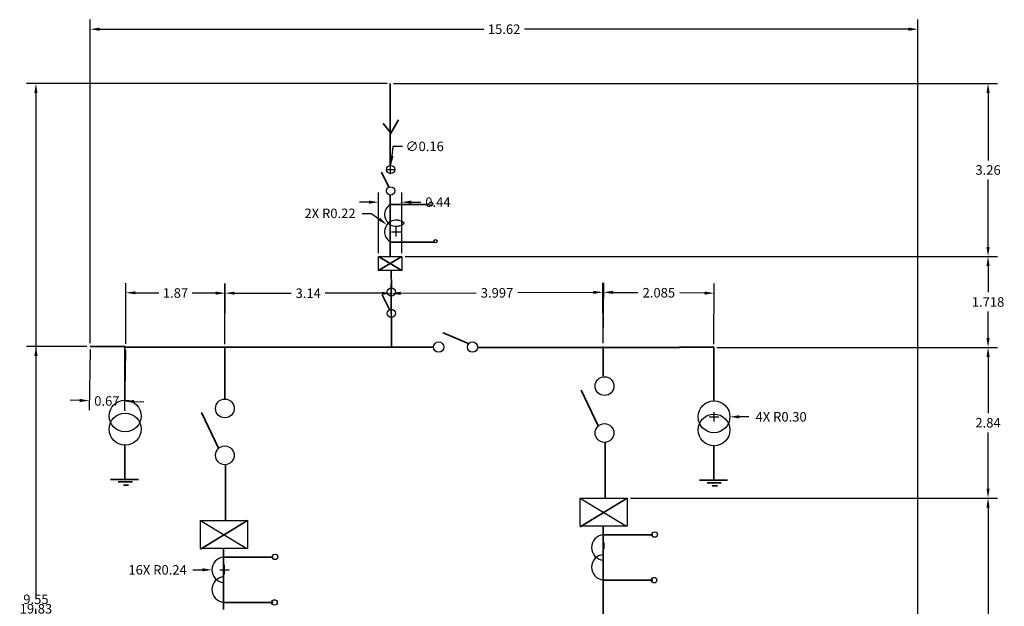
# Model space of a CAD drawing. Units: millimetres. Extents: x -4 to 31.8, y -11 to 11.2.
# Tile 2 of 2: x 13 to 31.6, y 0.1 to 11.2. Entities that reach past the tile are written whole.
import ezdxf

# ---------------------------------------------------------------- set-up
doc = ezdxf.new("R2010")
doc.units = ezdxf.units.MM
doc.header["$MEASUREMENT"] = 0
for name, color, linetype, lineweight in [('A-ANNO-DIMS', 2, 'Continuous', 18), ('E-ONEL-WIRE', 7, 'Continuous', 35), ('E-POWR-EQPM', 4, 'Continuous', 25)]:
    doc.layers.add(name, color=color, linetype=linetype, lineweight=lineweight)
doc.styles.get("Standard").update_dxf_attribs({"font": 'arial.ttf'})
doc.dimstyles.get("Standard").update_dxf_attribs({"dimtxt": 0.18, "dimasz": 0.18, "dimexe": 0.18, "dimexo": 0.0625, "dimgap": 0.09, "dimtad": 0, "dimtih": 1, "dimtoh": 1, "dimdec": 4, "dimzin": 0, "dimdsep": 46, "dimtxsty": 'Standard', "dimcen": 0.09, "dimadec": 0, "dimazin": 0, "dimtfac": 1, "dimtdec": 4, "dimtofl": 0, "dimtmove": 0, "dimatfit": 3, "dimfxl": 1, "dimtolj": 1, "dimtzin": 0, "dimarcsym": 0})

# ---------------------------------------------------------------- blocks, each defined once
blk = doc.blocks.new('CB-BREAKER')
blk.add_line((15.7, -7.316), (16.556, -7.832))
blk.add_lwpolyline([(15.685, -7.301), (16.571, -7.301), (16.571, -7.832), (15.685, -7.832)], close=True)
blk = doc.blocks.new('XFMR-AUX-SMALL')
for centre in [(26.095, 3.698), (26.095, 3.45)]:
    blk.add_circle(centre, 0.3)
blk = doc.blocks.new('*D7')
at = {"layer": 'A-ANNO-DIMS', "color": 0, "lineweight": -2, "transparency": 16777216}
for p, q in [((14.324, 5.091), (14.324, 11.195)), ((29.944, -4.451), (29.944, 11.195)), ((14.504, 11.015), (21.75, 11.015)), ((29.764, 11.015), (22.518, 11.015))]:
    blk.add_line(p, q, dxfattribs=at)
at = {"layer": 'A-ANNO-DIMS', "color": 0, "transparency": 16777216}
for points in [[(14.504, 11.045), (14.504, 10.985), (14.324, 11.015)], [(29.764, 11.045), (29.764, 10.985), (29.944, 11.015)]]:
    blk.add_solid(points, dxfattribs=at)
at = {"layer": 'Defpoints', "color": 0, "transparency": 16777216}
for p in [(29.944, 11.015), (14.324, 5.028), (29.944, -4.514)]:
    blk.add_point(p, dxfattribs=at)
at = {"layer": 'A-ANNO-DIMS', "color": 0, "transparency": 16777216, "insert": (22.134, 11.015), "char_height": 0.18, "attachment_point": 5}
blk.add_mtext('\\A1;15.62', dxfattribs=at)
blk = doc.blocks.new('*D8')
at = {"layer": 'A-ANNO-DIMS', "color": 0, "lineweight": -2, "transparency": 16777216}
for p, q in [((14.323, 4.966), (14.301, 3.823)), ((14.992, 4.952), (14.969, 3.81)), ((14.124, 4.007), (13.944, 4.01)), ((15.153, 3.987), (15.333, 3.983))]:
    blk.add_line(p, q, dxfattribs=at)
at = {"layer": 'A-ANNO-DIMS', "color": 0, "transparency": 16777216}
for points in [[(14.125, 4.037), (14.124, 3.977), (14.304, 4.003)], [(15.153, 4.017), (15.152, 3.957), (14.973, 3.99)]]:
    blk.add_solid(points, dxfattribs=at)
at = {"layer": 'Defpoints', "color": 0, "transparency": 16777216}
for p in [(14.324, 5.028), (14.993, 5.015), (14.304, 4.003)]:
    blk.add_point(p, dxfattribs=at)
at = {"layer": 'A-ANNO-DIMS', "color": 0, "transparency": 16777216, "insert": (14.638, 3.997), "char_height": 0.18, "attachment_point": 5}
blk.add_mtext('\\A1;0.67', dxfattribs=at)
blk = doc.blocks.new('*D9')
at = {"layer": 'A-ANNO-DIMS', "color": 0, "lineweight": -2, "transparency": 16777216}
for p, q in [((14.993, 5.077), (14.998, 6.22)), ((16.865, 5.069), (16.87, 6.212)), ((15.177, 6.039), (15.618, 6.037)), ((16.689, 6.033), (16.249, 6.035))]:
    blk.add_line(p, q, dxfattribs=at)
at = {"layer": 'A-ANNO-DIMS', "color": 0, "transparency": 16777216}
for points in [[(15.177, 6.069), (15.177, 6.009), (14.997, 6.04)], [(16.689, 6.063), (16.689, 6.003), (16.869, 6.032)]]:
    blk.add_solid(points, dxfattribs=at)
at = {"layer": 'Defpoints', "color": 0, "transparency": 16777216}
for p in [(16.869, 6.032), (14.993, 5.015), (16.865, 5.007)]:
    blk.add_point(p, dxfattribs=at)
at = {"layer": 'A-ANNO-DIMS', "color": 0, "transparency": 16777216, "insert": (15.933, 6.036), "char_height": 0.18, "attachment_point": 5}
blk.add_mtext('\\A1;1.87', dxfattribs=at)
blk = doc.blocks.new('*D10')
at = {"layer": 'A-ANNO-DIMS', "color": 0, "lineweight": -2, "transparency": 16777216}
for p, q in [((16.865, 5.069), (16.866, 6.212)), ((20.006, 5.066), (20.008, 6.208)), ((17.046, 6.032), (18.113, 6.03)), ((19.827, 6.029), (18.76, 6.03))]:
    blk.add_line(p, q, dxfattribs=at)
at = {"layer": 'A-ANNO-DIMS', "color": 0, "transparency": 16777216}
for points in [[(17.046, 6.062), (17.046, 6.002), (16.866, 6.032)], [(19.827, 6.059), (19.827, 5.999), (20.007, 6.028)]]:
    blk.add_solid(points, dxfattribs=at)
at = {"layer": 'Defpoints', "color": 0, "transparency": 16777216}
for p in [(20.007, 6.028), (16.865, 5.007), (20.006, 5.003)]:
    blk.add_point(p, dxfattribs=at)
at = {"layer": 'A-ANNO-DIMS', "color": 0, "transparency": 16777216, "insert": (18.437, 6.03), "char_height": 0.18, "attachment_point": 5}
blk.add_mtext('\\A1;3.14', dxfattribs=at)
blk = doc.blocks.new('*D11')
at = {"layer": 'A-ANNO-DIMS', "color": 0, "lineweight": -2, "transparency": 16777216}
for p, q in [((20.006, 5.066), (20, 6.208)), ((24.003, 5.086), (23.997, 6.228)), ((20.181, 6.029), (21.606, 6.036)), ((23.818, 6.047), (22.393, 6.04))]:
    blk.add_line(p, q, dxfattribs=at)
at = {"layer": 'A-ANNO-DIMS', "color": 0, "transparency": 16777216}
for points in [[(20.181, 6.059), (20.181, 5.999), (20.001, 6.028)], [(23.818, 6.077), (23.819, 6.017), (23.998, 6.048)]]:
    blk.add_solid(points, dxfattribs=at)
at = {"layer": 'Defpoints', "color": 0, "transparency": 16777216}
for p in [(23.998, 6.048), (24.003, 5.023), (20.006, 5.003)]:
    blk.add_point(p, dxfattribs=at)
at = {"layer": 'A-ANNO-DIMS', "color": 0, "transparency": 16777216, "insert": (22, 6.038), "char_height": 0.18, "attachment_point": 5}
blk.add_mtext('\\A1;3.997', dxfattribs=at)
blk = doc.blocks.new('*D12')
at = {"layer": 'A-ANNO-DIMS', "color": 0, "lineweight": -2, "transparency": 16777216}
for p, q in [((24.004, 5.086), (24.013, 6.228)), ((26.089, 5.069), (26.098, 6.212)), ((24.192, 6.047), (24.658, 6.043)), ((25.916, 6.033), (25.45, 6.037))]:
    blk.add_line(p, q, dxfattribs=at)
at = {"layer": 'A-ANNO-DIMS', "color": 0, "transparency": 16777216}
for points in [[(24.192, 6.077), (24.191, 6.017), (24.012, 6.048)], [(25.917, 6.063), (25.916, 6.003), (26.096, 6.032)]]:
    blk.add_solid(points, dxfattribs=at)
at = {"layer": 'Defpoints', "color": 0, "transparency": 16777216}
for p in [(26.096, 6.032), (24.003, 5.023), (26.088, 5.007)]:
    blk.add_point(p, dxfattribs=at)
at = {"layer": 'A-ANNO-DIMS', "color": 0, "transparency": 16777216, "insert": (25.054, 6.04), "char_height": 0.18, "attachment_point": 5}
blk.add_mtext('\\A1;2.085', dxfattribs=at)
blk = doc.blocks.new('*D13')
at = {"layer": 'A-ANNO-DIMS', "color": 0, "lineweight": -2, "transparency": 16777216}
for p, q in [((19.924, 9.99), (13.119, 9.99)), ((13.299, 9.81), (13.299, 0.256)), ((13.299, -9.661), (13.299, -0.108)), ((16.065, -9.841), (13.119, -9.841))]:
    blk.add_line(p, q, dxfattribs=at)
at = {"layer": 'A-ANNO-DIMS', "color": 0, "transparency": 16777216}
for points in [[(13.269, 9.81), (13.329, 9.81), (13.299, 9.99)], [(13.269, -9.661), (13.329, -9.661), (13.299, -9.841)]]:
    blk.add_solid(points, dxfattribs=at)
at = {"layer": 'Defpoints', "color": 0, "transparency": 16777216}
for p in [(13.299, 9.99), (19.987, 9.99), (16.127, -9.841)]:
    blk.add_point(p, dxfattribs=at)
at = {"layer": 'A-ANNO-DIMS', "color": 0, "transparency": 16777216, "insert": (13.299, 0.074), "char_height": 0.18, "attachment_point": 5}
blk.add_mtext('\\A1;19.83', dxfattribs=at)
blk = doc.blocks.new('*D14')
at = {"layer": 'A-ANNO-DIMS', "color": 0, "lineweight": -2, "transparency": 16777216}
for p, q in [((14.262, 5.028), (13.119, 5.028)), ((13.299, 4.848), (13.299, 0.435)), ((13.299, -4.342), (13.299, 0.071)), ((14.834, -4.522), (13.119, -4.522))]:
    blk.add_line(p, q, dxfattribs=at)
at = {"layer": 'A-ANNO-DIMS', "color": 0, "transparency": 16777216}
for points in [[(13.269, 4.848), (13.329, 4.848), (13.299, 5.028)], [(13.269, -4.342), (13.329, -4.342), (13.299, -4.522)]]:
    blk.add_solid(points, dxfattribs=at)
at = {"layer": 'Defpoints', "color": 0, "transparency": 16777216}
for p in [(13.299, 5.028), (14.324, 5.028), (14.897, -4.522)]:
    blk.add_point(p, dxfattribs=at)
at = {"layer": 'A-ANNO-DIMS', "color": 0, "transparency": 16777216, "insert": (13.299, 0.253), "char_height": 0.18, "attachment_point": 5}
blk.add_mtext('\\A1;9.55', dxfattribs=at)
blk = doc.blocks.new('*D15')
at = {"layer": 'A-ANNO-DIMS', "color": 0, "lineweight": -2, "transparency": 16777216}
for p, q in [((20.049, 9.99), (31.446, 9.99)), ((31.266, 9.81), (31.266, 8.539)), ((31.266, 6.905), (31.266, 8.175)), ((20.264, 6.725), (31.446, 6.725))]:
    blk.add_line(p, q, dxfattribs=at)
at = {"layer": 'A-ANNO-DIMS', "color": 0, "transparency": 16777216}
for points in [[(31.236, 9.81), (31.296, 9.81), (31.266, 9.99)], [(31.236, 6.905), (31.296, 6.905), (31.266, 6.725)]]:
    blk.add_solid(points, dxfattribs=at)
at = {"layer": 'Defpoints', "color": 0, "transparency": 16777216}
for p in [(19.987, 9.99), (31.266, 9.99), (20.202, 6.725)]:
    blk.add_point(p, dxfattribs=at)
at = {"layer": 'A-ANNO-DIMS', "color": 0, "transparency": 16777216, "insert": (31.266, 8.357), "char_height": 0.18, "attachment_point": 5}
blk.add_mtext('\\A1;3.26', dxfattribs=at)
blk = doc.blocks.new('*D16')
at = {"layer": 'A-ANNO-DIMS', "color": 0, "lineweight": -2, "transparency": 16777216}
for p, q in [((20.264, 6.725), (31.446, 6.725)), ((31.266, 6.545), (31.266, 6.048)), ((31.266, 5.187), (31.266, 5.684)), ((26.151, 5.007), (31.446, 5.007))]:
    blk.add_line(p, q, dxfattribs=at)
at = {"layer": 'A-ANNO-DIMS', "color": 0, "transparency": 16777216}
for points in [[(31.236, 6.545), (31.296, 6.545), (31.266, 6.725)], [(31.236, 5.187), (31.296, 5.187), (31.266, 5.007)]]:
    blk.add_solid(points, dxfattribs=at)
at = {"layer": 'Defpoints', "color": 0, "transparency": 16777216}
for p in [(20.202, 6.725), (31.266, 6.725), (26.088, 5.007)]:
    blk.add_point(p, dxfattribs=at)
at = {"layer": 'A-ANNO-DIMS', "color": 0, "transparency": 16777216, "insert": (31.266, 5.866), "char_height": 0.18, "attachment_point": 5}
blk.add_mtext('\\A1;1.718', dxfattribs=at)
blk = doc.blocks.new('*D17')
at = {"layer": 'A-ANNO-DIMS', "color": 0, "lineweight": -2, "transparency": 16777216}
for p, q in [((26.151, 5.007), (31.446, 5.007)), ((31.266, 4.827), (31.266, 3.767)), ((31.266, 2.344), (31.266, 3.404)), ((24.519, 2.164), (31.446, 2.164))]:
    blk.add_line(p, q, dxfattribs=at)
at = {"layer": 'A-ANNO-DIMS', "color": 0, "transparency": 16777216}
for points in [[(31.236, 4.827), (31.296, 4.827), (31.266, 5.007)], [(31.236, 2.344), (31.296, 2.344), (31.266, 2.164)]]:
    blk.add_solid(points, dxfattribs=at)
at = {"layer": 'Defpoints', "color": 0, "transparency": 16777216}
for p in [(26.088, 5.007), (31.266, 5.007), (24.456, 2.164)]:
    blk.add_point(p, dxfattribs=at)
at = {"layer": 'A-ANNO-DIMS', "color": 0, "transparency": 16777216, "insert": (31.266, 3.586), "char_height": 0.18, "attachment_point": 5}
blk.add_mtext('\\A1;2.84', dxfattribs=at)
blk = doc.blocks.new('*D18')
at = {"layer": 'A-ANNO-DIMS', "color": 0, "lineweight": -2, "transparency": 16777216}
for p, q in [((24.519, 2.164), (31.446, 2.164)), ((31.266, 1.984), (31.266, -0.248)), ((31.266, -2.844), (31.266, -0.612)), ((24.43, -3.024), (31.446, -3.024))]:
    blk.add_line(p, q, dxfattribs=at)
at = {"layer": 'A-ANNO-DIMS', "color": 0, "transparency": 16777216}
for points in [[(31.236, 1.984), (31.296, 1.984), (31.266, 2.164)], [(31.236, -2.844), (31.296, -2.844), (31.266, -3.024)]]:
    blk.add_solid(points, dxfattribs=at)
at = {"layer": 'Defpoints', "color": 0, "transparency": 16777216}
for p in [(24.456, 2.164), (31.266, 2.164), (24.367, -3.024)]:
    blk.add_point(p, dxfattribs=at)
at = {"layer": 'A-ANNO-DIMS', "color": 0, "transparency": 16777216, "insert": (31.266, -0.43), "char_height": 0.18, "attachment_point": 5}
blk.add_mtext('\\A1;5.188', dxfattribs=at)
blk = doc.blocks.new('*D32')
at = {"layer": 'A-ANNO-DIMS', "color": 0, "lineweight": -2, "transparency": 16777216}
for p, q in [((19.765, 6.788), (19.765, 7.93)), ((20.202, 6.788), (20.202, 7.93)), ((19.585, 7.75), (19.405, 7.75)), ((20.382, 7.75), (20.562, 7.75))]:
    blk.add_line(p, q, dxfattribs=at)
at = {"layer": 'A-ANNO-DIMS', "color": 0, "transparency": 16777216}
for points in [[(19.585, 7.78), (19.585, 7.72), (19.765, 7.75)], [(20.382, 7.78), (20.382, 7.72), (20.202, 7.75)]]:
    blk.add_solid(points, dxfattribs=at)
at = {"layer": 'Defpoints', "color": 0, "transparency": 16777216}
for p in [(20.202, 7.75), (19.765, 6.725), (20.202, 6.725)]:
    blk.add_point(p, dxfattribs=at)
at = {"layer": 'A-ANNO-DIMS', "color": 0, "transparency": 16777216, "insert": (20.885, 7.75), "char_height": 0.18, "attachment_point": 5}
blk.add_mtext('\\A1;0.44', dxfattribs=at)
blk = doc.blocks.new('*D35')
at = {"layer": 'A-ANNO-DIMS', "color": 0, "lineweight": -2, "transparency": 16777216}
for p, q in [((26.095, 3.608), (26.095, 3.788)), ((26.005, 3.698), (26.185, 3.698)), ((26.754, 3.698), (26.574, 3.698))]:
    blk.add_line(p, q, dxfattribs=at)
at = {"layer": 'A-ANNO-DIMS', "color": 0, "transparency": 16777216}
blk.add_solid([(26.574, 3.728), (26.574, 3.668), (26.394, 3.698)], dxfattribs=at)
at = {"layer": 'Defpoints', "color": 0, "transparency": 16777216}
for p in [(26.095, 3.698), (26.394, 3.698)]:
    blk.add_point(p, dxfattribs=at)
at = {"layer": 'A-ANNO-DIMS', "color": 0, "transparency": 16777216, "insert": (27.361, 3.698), "char_height": 0.18, "attachment_point": 5}
blk.add_mtext('\\A1;4X R0.30', dxfattribs=at)
blk = doc.blocks.new('*D37')
at = {"layer": 'A-ANNO-DIMS', "color": 0, "lineweight": -2, "transparency": 16777216}
for p, q in [((16.259, 0.808), (16.439, 0.809)), ((16.768, 0.809), (16.948, 0.809)), ((16.858, 0.719), (16.858, 0.899))]:
    blk.add_line(p, q, dxfattribs=at)
at = {"layer": 'A-ANNO-DIMS', "color": 0, "transparency": 16777216}
blk.add_solid([(16.439, 0.839), (16.44, 0.779), (16.619, 0.809)], dxfattribs=at)
at = {"layer": 'Defpoints', "color": 0, "transparency": 16777216}
for p in [(16.619, 0.809), (16.858, 0.809)]:
    blk.add_point(p, dxfattribs=at)
at = {"layer": 'A-ANNO-DIMS', "color": 0, "transparency": 16777216, "insert": (15.595, 0.808), "char_height": 0.18, "attachment_point": 5}
blk.add_mtext('\\A1;16X R0.24', dxfattribs=at)
blk = doc.blocks.new('*D38')
at = {"layer": 'A-ANNO-DIMS', "color": 0, "lineweight": -2, "transparency": 16777216}
for p, q in [((19.453, 7.538), (19.633, 7.538)), ((19.633, 7.538), (19.777, 7.431)), ((20.098, 7.102), (20.098, 7.282)), ((20.008, 7.192), (20.188, 7.192))]:
    blk.add_line(p, q, dxfattribs=at)
at = {"layer": 'A-ANNO-DIMS', "color": 0, "transparency": 16777216}
blk.add_solid([(19.795, 7.455), (19.759, 7.407), (19.922, 7.323)], dxfattribs=at)
at = {"layer": 'Defpoints', "color": 0, "transparency": 16777216}
for p in [(19.922, 7.323), (20.098, 7.192)]:
    blk.add_point(p, dxfattribs=at)
at = {"layer": 'A-ANNO-DIMS', "color": 0, "transparency": 16777216, "insert": (18.849, 7.538), "char_height": 0.18, "attachment_point": 5}
blk.add_mtext('\\A1;2X R0.22', dxfattribs=at)
blk = doc.blocks.new('*D41')
at = {"layer": 'A-ANNO-DIMS', "color": 0, "lineweight": -2, "transparency": 16777216}
for p, q in [((20.034, 8.803), (20.017, 8.623)), ((20.214, 8.803), (20.034, 8.803)), ((19.903, 8.366), (20.083, 8.366)), ((19.993, 8.276), (19.993, 8.456))]:
    blk.add_line(p, q, dxfattribs=at)
at = {"layer": 'A-ANNO-DIMS', "color": 0, "transparency": 16777216}
blk.add_solid([(19.987, 8.626), (20.047, 8.621), (20, 8.444)], dxfattribs=at)
at = {"layer": 'Defpoints', "color": 0, "transparency": 16777216}
for p in [(20, 8.444), (19.986, 8.288)]:
    blk.add_point(p, dxfattribs=at)
at = {"layer": 'A-ANNO-DIMS', "color": 0, "transparency": 16777216, "insert": (20.635, 8.803), "char_height": 0.18, "attachment_point": 5}
blk.add_mtext('\\A1;∅0.16', dxfattribs=at)

msp = doc.modelspace()

# ---------------------------------------------------------------- linework, layer by layer
at = {"layer": 'E-ONEL-WIRE'}
for p, q in [((19.9867, 9.9896), (19.9867, 8.4395)), ((19.9921, 9.0419), (20.1412, 9.3055)), ((20.1412, 9.3055), (20.1412, 9.3055)), ((19.9921, 9.0649), (19.8545, 9.2367)), ((19.9867, 8.4395), (19.9867, 8.4656)), ((19.9671, 8.0211), (19.8172, 8.3141)), ((19.9866, 7.8778), (19.9866, 6.9269)), ((19.9857, 7.7026), (20.716, 7.7026)), ((19.9866, 6.953), (19.9866, 6.725)), ((19.9902, 6.9954), (20.8235, 6.9954)), ((20.8235, 6.9954), (20.7205, 6.9954)), ((20.2018, 6.458), (19.765, 6.725)), ((20.2018, 6.725), (19.765, 6.458)), ((20.0062, 6.1325), (19.9997, 6.458)), ((19.9997, 6.1276), (19.9997, 6.1536)), ((19.9801, 5.7091), (19.8302, 6.0022)), ((20.0062, 5.5723), (20.0062, 5.0034)), ((20.984, 5.2816), (20.9775, 5.2751)), ((21.473, 5.0732), (20.984, 5.2816)), ((14.3245, 5.0281), (14.9829, 5.0281)), ((14.9764, 5.0216), (14.9764, 4.0121)), ((24.0035, 4.4733), (24.0035, 5.0233)), ((14.9929, 5.0149), (20.8012, 5.0149)), ((16.8647, 5.0069), (16.8647, 4.033)), ((21.6359, 5.0081), (25.456, 5.0081)), ((25.4365, 5.0134), (26.0949, 5.0134)), ((26.0884, 5.0069), (26.0884, 3.9974)), ((23.9102, 3.5249), (23.5853, 4.2037)), ((16.7465, 3.1035), (16.4216, 3.7822)), ((14.9764, 3.1655), (14.9764, 2.5142)), ((24.0428, 3.2266), (24.0428, 2.1643)), ((26.0884, 3.1508), (26.0884, 2.4995)), ((16.8791, 2.8052), (16.8791, 1.7429)), ((14.7091, 2.5142), (15.2371, 2.5142)), ((14.8525, 2.4686), (15.1198, 2.4686)), ((25.8211, 2.4995), (26.3491, 2.4995)), ((25.9645, 2.4539), (26.2318, 2.4539)), ((14.9503, 2.41), (15.0481, 2.41)), ((24.0428, 2.3266), (24.0428, 2.3856)), ((26.0623, 2.3953), (26.1601, 2.3953)), ((24.4564, 2.1643), (23.5703, 1.6184)), ((16.8791, 1.9052), (16.8791, 1.9642)), ((17.2927, 1.7429), (16.4065, 1.1969)), ((24.0042, 1.626), (24.0042, 0.4812)), ((24.01, 1.4691), (24.9407, 1.4691)), ((24.0133, 1.2052), (24.0133, 1.3233)), ((24.0133, 1.3233), (24.0133, 1.3233)), ((16.8405, 1.2045), (16.8405, 0.0598)), ((16.8463, 1.0476), (17.777, 1.0476)), ((16.8496, 0.7838), (16.8496, 0.9018)), ((16.8496, 0.9018), (16.8496, 0.9018)), ((24.01, 0.6149), (24.9407, 0.6149)), ((24.0041, 0.5211), (24.0041, -0.2518)), ((24.0042, 0.4812), (24.0042, 0.4986)), ((16.8463, 0.1934), (17.777, 0.1934))]:
    msp.add_line(p, q, dxfattribs=at)
at = {"layer": 'E-POWR-EQPM'}
msp.add_lwpolyline([(19.765, 6.725), (20.2018, 6.725), (20.2018, 6.458), (19.765, 6.458)], close=True, dxfattribs=at)
for centre, radius in [((19.9932, 8.3662), 0.0782), ((19.9932, 7.9624), 0.0782), ((20.7518, 7.716), 0.0358), ((20.837, 7.0133), 0.0314), ((20.0062, 6.0543), 0.0782), ((20.0062, 5.6505), 0.0782), ((20.8989, 5.0149), 0.0977), ((21.5385, 5.0149), 0.0977), ((24.0284, 4.2774), 0.1771), ((16.8647, 3.856), 0.1771), ((24.0284, 3.3922), 0.1771), ((16.8647, 2.9707), 0.1771), ((24.9756, 1.4749), 0.0523), ((17.8119, 1.0534), 0.0523), ((24.9639, 0.6149), 0.0523), ((17.8002, 0.1934), 0.0523)]:
    msp.add_circle(centre, radius, dxfattribs=at)
for centre, radius, start, end in [((20.0977, 7.5146), 0.2193, 120.43765, 312.71863), ((20.0977, 7.1923), 0.2193, 47.28137, 239.56235), ((24.0217, 1.2308), 0.2385, 94.19612, 265.80388), ((16.858, 0.8094), 0.2385, 94.19612, 265.80388), ((24.0217, 0.8589), 0.2385, 94.19612, 265.80388), ((16.858, 0.4375), 0.2385, 94.19612, 265.80388)]:
    msp.add_arc(centre, radius, start, end, dxfattribs=at)

# ---------------------------------------------------------------- block references
for name, p in [('XFMR-AUX-SMALL', (-11.112, 0.0147)), ('XFMR-AUX-SMALL', (0, 0)), ('CB-BREAKER', (7.8853, 9.4655)), ('CB-BREAKER', (0.7216, 9.0441))]:
    msp.add_blockref(name, p, dxfattribs=at)

# ---------------------------------------------------------------- dimensions: what is measured, and where the dimension line sits
at = {"layer": 'A-ANNO-DIMS'}
for base, p1, p2, picture, middle in [((29.9436, 11.0146), (14.3245, 5.0281), (29.9436, -4.5139), '*D7', (22.134, 11.0146)), ((20.2018, 7.75), (19.765, 6.725), (20.2018, 6.725), '*D32', (20.8852, 7.75))]:
    dim = msp.add_linear_dim(base=base, p1=p1, p2=p2, dimstyle='Standard', override={"dimdec": 2, "dimlfac": 1, "dimrnd": 0, "dimzin": 0, "dimdsep": 46, "dimlunit": 2}, dxfattribs=at)
    dim.commit()
    dim.dimension.update_dxf_attribs({"geometry": picture, "text_midpoint": middle})
for base, p1, p2, angle, override, picture, middle in [((13.2995, 9.9896), (16.127, -9.8408), (19.9867, 9.9896), 90, {"dimdec": 2, "dimlfac": 1, "dimrnd": 0, "dimzin": 0, "dimdsep": 46, "dimlunit": 2}, '*D13', (13.2995, 0.0744)), ((31.2659, 9.9896), (20.2018, 6.725), (19.9867, 9.9896), 90, {"dimdec": 2, "dimlfac": 1, "dimrnd": 0, "dimzin": 0, "dimdsep": 46, "dimlunit": 2}, '*D15', (31.2659, 8.3573)), ((31.2659, 6.725), (26.0884, 5.0069), (20.2018, 6.725), 90, {"dimdec": 3, "dimlfac": 1, "dimrnd": 0, "dimzin": 0, "dimdsep": 46, "dimlunit": 2}, '*D16', (31.2659, 5.866)), ((16.8691, 6.0318), (14.9929, 5.0149), (16.8647, 5.0069), 359.75319, {"dimdec": 2, "dimlfac": 1, "dimrnd": 0, "dimzin": 0, "dimdsep": 46, "dimlunit": 2}, '*D9', (15.9332, 6.0359)), ((20.0073, 6.0284), (16.8647, 5.0069), (20.0062, 5.0034), 359.93701, {"dimdec": 2, "dimlfac": 1, "dimrnd": 0, "dimzin": 0, "dimdsep": 46, "dimlunit": 2}, '*D10', (18.4366, 6.0301)), ((23.9984, 6.0483), (20.0062, 5.0034), (24.0035, 5.0233), 0.28523, {"dimdec": 3, "dimlfac": 1, "dimrnd": 0, "dimzin": 0, "dimdsep": 46, "dimlunit": 2}, '*D11', (21.9997, 6.0383)), ((26.0964, 6.0319), (24.0035, 5.0233), (26.0884, 5.0069), 359.54893, {"dimdec": 3, "dimlfac": 1, "dimrnd": 0, "dimzin": 0, "dimdsep": 46, "dimlunit": 2}, '*D12', (25.054, 6.0401)), ((13.2995, 5.0281), (14.8965, -4.522), (14.3245, 5.0281), 90, {"dimdec": 2, "dimlfac": 1, "dimrnd": 0, "dimzin": 0, "dimdsep": 46, "dimlunit": 2}, '*D14', (13.2995, 0.2531)), ((14.3042, 4.0033), (14.9929, 5.0149), (14.3245, 5.0281), 178.867, {"dimdec": 2, "dimlfac": 1, "dimrnd": 0, "dimzin": 0, "dimdsep": 46, "dimlunit": 2}, '*D8', (14.6384, 3.9967)), ((31.2659, 5.0069), (24.4564, 2.1643), (26.0884, 5.0069), 90, {"dimdec": 2, "dimlfac": 1, "dimrnd": 0, "dimzin": 0, "dimdsep": 46, "dimlunit": 2}, '*D17', (31.2659, 3.5856)), ((31.2659, 2.1643), (24.3672, -3.0241), (24.4564, 2.1643), 90, {"dimdec": 3, "dimlfac": 1, "dimrnd": 0, "dimzin": 0, "dimdsep": 46, "dimlunit": 2}, '*D18', (31.2659, -0.4299))]:
    dim = msp.add_linear_dim(base=base, p1=p1, p2=p2, angle=angle, dimstyle='Standard', override=override, dxfattribs=at)
    dim.commit()
    dim.dimension.update_dxf_attribs({"geometry": picture, "text_midpoint": middle})
dim = msp.add_diameter_dim_2p(p1=(19.9859, 8.2883), p2=(20.0004, 8.4441), dimstyle='Standard', override={"dimdec": 2, "dimlfac": 1, "dimrnd": 0, "dimzin": 0, "dimdsep": 46, "dimlunit": 2}, dxfattribs=at)
dim.commit()
dim.dimension.update_dxf_attribs({"geometry": '*D41', "text_midpoint": (20.6353, 8.8026), "dimtype": 163})
for center, mpoint, text, picture, middle in [((20.0977, 7.1923), (19.9217, 7.3232), '2X <>', '*D38', (18.8489, 7.538)), ((26.0949, 3.6978), (26.3945, 3.698), '4X <>', '*D35', (27.3611, 3.6982)), ((16.858, 0.8094), (16.6195, 0.809), '16X <>', '*D37', (15.5951, 0.8084))]:
    dim = msp.add_radius_dim(center=center, mpoint=mpoint, text=text, dimstyle='Standard', override={"dimdec": 2, "dimlfac": 1, "dimrnd": 0, "dimzin": 0, "dimdsep": 46, "dimlunit": 2}, dxfattribs=at)
    dim.commit()
    dim.dimension.update_dxf_attribs({"geometry": picture, "text_midpoint": middle})

doc.saveas('drawing.dxf')
